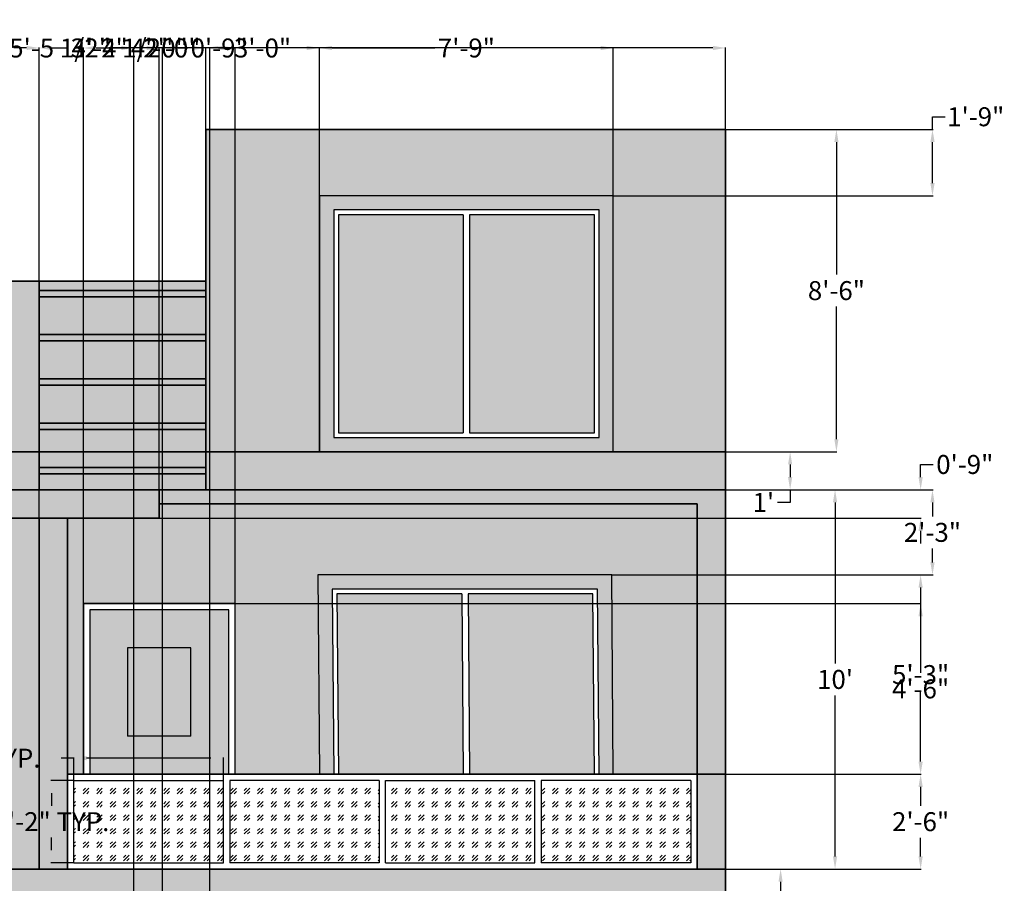
# Model space of a CAD drawing. Units: inches. Extents: x 23 to 640, y 58 to 516.
# Tile 4 of 4: x 328 to 639, y 243 to 516. Entities that reach past the tile are written whole.
import ezdxf

# ---------------------------------------------------------------- set-up
doc = ezdxf.new("R2010")
doc.units = ezdxf.units.IN
doc.header["$MEASUREMENT"] = 0
for name, color, linetype, lineweight in [('A-ANNO-DIMS', 2, 'Continuous', 18), ('A-DOOR', 3, 'Continuous', 25), ('A-ELEV', 7, 'Continuous', 35), ('A-ELEV-PATT', 252, 'Continuous', 13), ('A-GLAZ', 4, 'Continuous', 25)]:
    doc.layers.add(name, color=color, linetype=linetype, lineweight=lineweight)
doc.styles.get("Standard").update_dxf_attribs({"font": 'arial.ttf'})
doc.dimstyles.get("Standard").update_dxf_attribs({"dimtxt": 6, "dimasz": 4, "dimexe": 0.18, "dimexo": 0.0625, "dimgap": 2, "dimtad": 0, "dimtih": 1, "dimtoh": 1, "dimdec": 0, "dimzin": 0, "dimdsep": 46, "dimlunit": 3, "dimtxsty": 'Standard', "dimcen": 2, "dimadec": 0, "dimazin": 0, "dimtfac": 1, "dimtdec": 0, "dimtofl": 0, "dimtmove": 0, "dimatfit": 3, "dimfxl": 1, "dimtolj": 1, "dimtzin": 0, "dimarcsym": 0})

# ---------------------------------------------------------------- blocks, each defined once
blk = doc.blocks.new('*D6')
at = {"layer": 'A-ANNO-DIMS', "color": 0, "lineweight": -2, "transparency": 16777216}
for p, q in [((551.19, 481.68), (586.41, 481.68)), ((586.23, 477.68), (586.23, 435.74)), ((586.23, 383.68), (586.23, 425.62)), ((551.19, 379.68), (586.41, 379.68))]:
    blk.add_line(p, q, dxfattribs=at)
at = {"layer": 'A-ANNO-DIMS', "color": 0, "transparency": 16777216}
for points in [[(585.57, 477.68), (586.9, 477.68), (586.23, 481.68)], [(585.57, 383.68), (586.9, 383.68), (586.23, 379.68)]]:
    blk.add_solid(points, dxfattribs=at)
at = {"layer": 'Defpoints', "color": 0, "transparency": 16777216}
for p in [(551.13, 481.68), (551.13, 379.68), (586.23, 379.68)]:
    blk.add_point(p, dxfattribs=at)
at = {"layer": 'A-ANNO-DIMS', "color": 0, "transparency": 16777216, "insert": (586.23, 430.68), "char_height": 6, "attachment_point": 5}
blk.add_mtext('\\A1;8\'-6"', dxfattribs=at)
blk = doc.blocks.new('*D7')
at = {"layer": 'A-ANNO-DIMS', "color": 0, "lineweight": -2, "transparency": 16777216}
for p, q in [((551.19, 379.68), (571.76, 379.68)), ((571.58, 375.68), (571.58, 371.68)), ((551.19, 367.68), (571.76, 367.68)), ((571.58, 367.68), (571.58, 363.68)), ((571.58, 363.68), (567.58, 363.68))]:
    blk.add_line(p, q, dxfattribs=at)
at = {"layer": 'A-ANNO-DIMS', "color": 0, "transparency": 16777216}
for points in [[(570.92, 375.68), (572.25, 375.68), (571.58, 379.68)], [(570.92, 371.68), (572.25, 371.68), (571.58, 367.68)]]:
    blk.add_solid(points, dxfattribs=at)
at = {"layer": 'Defpoints', "color": 0, "transparency": 16777216}
for p in [(551.13, 379.68), (551.13, 367.68), (571.58, 367.68)]:
    blk.add_point(p, dxfattribs=at)
at = {"layer": 'A-ANNO-DIMS', "color": 0, "transparency": 16777216, "insert": (563.11, 363.68), "char_height": 6, "attachment_point": 5}
blk.add_mtext("\\A1;1'", dxfattribs=at)
blk = doc.blocks.new('*D8')
at = {"layer": 'A-ANNO-DIMS', "color": 0, "lineweight": -2, "transparency": 16777216}
for p, q in [((551.19, 367.68), (585.98, 367.68)), ((585.8, 363.68), (585.8, 312.74)), ((585.8, 251.68), (585.8, 302.62)), ((551.19, 247.68), (585.98, 247.68))]:
    blk.add_line(p, q, dxfattribs=at)
at = {"layer": 'A-ANNO-DIMS', "color": 0, "transparency": 16777216}
for points in [[(585.13, 363.68), (586.47, 363.68), (585.8, 367.68)], [(585.13, 251.68), (586.47, 251.68), (585.8, 247.68)]]:
    blk.add_solid(points, dxfattribs=at)
at = {"layer": 'Defpoints', "color": 0, "transparency": 16777216}
for p in [(551.13, 367.68), (551.13, 247.68), (585.8, 247.68)]:
    blk.add_point(p, dxfattribs=at)
at = {"layer": 'A-ANNO-DIMS', "color": 0, "transparency": 16777216, "insert": (585.8, 307.68), "char_height": 6, "attachment_point": 5}
blk.add_mtext("\\A1;10'", dxfattribs=at)
blk = doc.blocks.new('*D9')
at = {"layer": 'A-ANNO-DIMS', "color": 0, "lineweight": -2, "transparency": 16777216}
for p, q in [((551.19, 247.68), (568.75, 247.68)), ((568.57, 243.68), (568.57, 239.68)), ((551.19, 235.68), (568.75, 235.68)), ((568.57, 235.68), (568.57, 231.68)), ((568.57, 231.68), (564.57, 231.68))]:
    blk.add_line(p, q, dxfattribs=at)
at = {"layer": 'A-ANNO-DIMS', "color": 0, "transparency": 16777216}
for points in [[(567.9, 243.68), (569.23, 243.68), (568.57, 247.68)], [(567.9, 239.68), (569.23, 239.68), (568.57, 235.68)]]:
    blk.add_solid(points, dxfattribs=at)
at = {"layer": 'Defpoints', "color": 0, "transparency": 16777216}
for p in [(551.13, 247.68), (551.13, 235.68), (568.57, 235.68)]:
    blk.add_point(p, dxfattribs=at)
at = {"layer": 'A-ANNO-DIMS', "color": 0, "transparency": 16777216, "insert": (560.09, 231.68), "char_height": 6, "attachment_point": 5}
blk.add_mtext("\\A1;1'", dxfattribs=at)
blk = doc.blocks.new('WIN-SLIDING-2P')
for p, q in [((45.5, 75), (45.5, 6)), ((47.5, 75), (47.5, 6))]:
    blk.add_line(p, q)
for points in [[(93, 81), (0, 81), (0, 0), (93, 0)], [(88.5, 76.5), (4.5, 76.5), (4.5, 4.5), (88.5, 4.5)]]:
    blk.add_lwpolyline(points, close=True)
for points in [[(45.5, 75), (6, 75), (6, 6), (45.5, 6)], [(47.5, 6), (87, 6), (87, 75), (47.5, 75)]]:
    blk.add_lwpolyline(points)
blk = doc.blocks.new('RAIL-GLASS-PANEL')
for p, q in [((47.3, 26), (0, 26)), ((0, 26), (0, 0)), ((47.3, 26), (47.3, 0)), ((47.3, 0), (0, 0))]:
    blk.add_line(p, q)
blk = doc.blocks.new('*D13')
at = {"layer": 'A-ANNO-DIMS', "color": 0, "lineweight": -2, "transparency": 16777216}
for p, q in [((344.93, 282.78), (340.93, 282.78)), ((344.93, 275.74), (344.93, 282.96)), ((388.23, 282.78), (348.93, 282.78)), ((392.23, 275.74), (392.23, 282.96))]:
    blk.add_line(p, q, dxfattribs=at)
at = {"layer": 'A-ANNO-DIMS', "color": 0, "transparency": 16777216}
for points in [[(348.93, 283.44), (348.93, 282.11), (344.93, 282.78)], [(388.23, 283.44), (388.23, 282.11), (392.23, 282.78)]]:
    blk.add_solid(points, dxfattribs=at)
at = {"layer": 'Defpoints', "color": 0, "transparency": 16777216}
for p in [(344.93, 282.78), (344.93, 275.68), (392.23, 275.68)]:
    blk.add_point(p, dxfattribs=at)
at = {"layer": 'A-ANNO-DIMS', "color": 0, "transparency": 16777216, "insert": (263.39, 282.78), "char_height": 6, "attachment_point": 5}
blk.add_mtext('\\A1;GLASS RAILING PANEL 3\'-11 1/2" TYP.', dxfattribs=at)
blk = doc.blocks.new('*D14')
at = {"layer": 'A-ANNO-DIMS', "color": 0, "lineweight": -2, "transparency": 16777216}
for p, q in [((344.87, 275.68), (337.65, 275.68)), ((337.83, 271.68), (337.83, 267.7)), ((337.83, 253.68), (337.83, 257.67)), ((344.87, 249.68), (337.65, 249.68))]:
    blk.add_line(p, q, dxfattribs=at)
at = {"layer": 'A-ANNO-DIMS', "color": 0, "transparency": 16777216}
for points in [[(337.17, 271.68), (338.5, 271.68), (337.83, 275.68)], [(337.17, 253.68), (338.5, 253.68), (337.83, 249.68)]]:
    blk.add_solid(points, dxfattribs=at)
at = {"layer": 'Defpoints', "color": 0, "transparency": 16777216}
for p in [(344.93, 275.68), (337.83, 249.68), (344.93, 249.68)]:
    blk.add_point(p, dxfattribs=at)
at = {"layer": 'A-ANNO-DIMS', "color": 0, "transparency": 16777216, "insert": (337.83, 262.68), "char_height": 6, "attachment_point": 5}
blk.add_mtext('\\A1;2\'-2" TYP.', dxfattribs=at)
blk = doc.blocks.new('*D18')
at = {"layer": 'A-ANNO-DIMS', "color": 0, "lineweight": -2, "transparency": 16777216}
for p, q in [((297.93, 433.74), (297.93, 507.61)), ((301.93, 507.43), (305.96, 507.43)), ((329.93, 507.43), (325.9, 507.43)), ((333.93, 433.74), (333.93, 507.61))]:
    blk.add_line(p, q, dxfattribs=at)
at = {"layer": 'A-ANNO-DIMS', "color": 0, "transparency": 16777216}
for points in [[(301.93, 508.1), (301.93, 506.76), (297.93, 507.43)], [(329.93, 508.1), (329.93, 506.76), (333.93, 507.43)]]:
    blk.add_solid(points, dxfattribs=at)
at = {"layer": 'Defpoints', "color": 0, "transparency": 16777216}
for p in [(333.93, 507.43), (297.93, 433.68), (333.93, 433.68)]:
    blk.add_point(p, dxfattribs=at)
at = {"layer": 'A-ANNO-DIMS', "color": 0, "transparency": 16777216, "insert": (315.93, 507.43), "char_height": 6, "attachment_point": 5}
blk.add_mtext('\\A1;3\'-0"', dxfattribs=at)
blk = doc.blocks.new('*D19')
at = {"layer": 'A-ANNO-DIMS', "color": 0, "lineweight": -2, "transparency": 16777216}
for p, q in [((333.93, 433.74), (333.93, 507.61)), ((337.93, 507.43), (343.19, 507.43)), ((382.63, 507.43), (377.36, 507.43)), ((386.63, 481.74), (386.63, 507.61))]:
    blk.add_line(p, q, dxfattribs=at)
at = {"layer": 'A-ANNO-DIMS', "color": 0, "transparency": 16777216}
for points in [[(337.93, 508.1), (337.93, 506.76), (333.93, 507.43)], [(382.63, 508.1), (382.63, 506.76), (386.63, 507.43)]]:
    blk.add_solid(points, dxfattribs=at)
at = {"layer": 'Defpoints', "color": 0, "transparency": 16777216}
for p in [(386.63, 507.43), (386.63, 481.68), (333.93, 433.68)]:
    blk.add_point(p, dxfattribs=at)
at = {"layer": 'A-ANNO-DIMS', "color": 0, "transparency": 16777216, "insert": (360.28, 507.43), "char_height": 6, "attachment_point": 5}
blk.add_mtext('\\A1;4\'-4 1/2"', dxfattribs=at)
blk = doc.blocks.new('*D20')
at = {"layer": 'A-ANNO-DIMS', "color": 0, "lineweight": -2, "transparency": 16777216}
for p, q in [((386.63, 374.82), (386.63, 507.61)), ((390.63, 507.43), (394.66, 507.43)), ((418.63, 507.43), (414.6, 507.43)), ((422.63, 379.74), (422.63, 507.61))]:
    blk.add_line(p, q, dxfattribs=at)
at = {"layer": 'A-ANNO-DIMS', "color": 0, "transparency": 16777216}
for points in [[(390.63, 508.1), (390.63, 506.76), (386.63, 507.43)], [(418.63, 508.1), (418.63, 506.76), (422.63, 507.43)]]:
    blk.add_solid(points, dxfattribs=at)
at = {"layer": 'Defpoints', "color": 0, "transparency": 16777216}
for p in [(422.63, 507.43), (422.63, 379.68), (386.63, 374.76)]:
    blk.add_point(p, dxfattribs=at)
at = {"layer": 'A-ANNO-DIMS', "color": 0, "transparency": 16777216, "insert": (404.63, 507.43), "char_height": 6, "attachment_point": 5}
blk.add_mtext('\\A1;3\'-0"', dxfattribs=at)
blk = doc.blocks.new('*D21')
at = {"layer": 'A-ANNO-DIMS', "color": 0, "lineweight": -2, "transparency": 16777216}
for p, q in [((422.63, 379.74), (422.63, 507.61)), ((426.63, 507.43), (459.18, 507.43)), ((511.63, 507.43), (479.08, 507.43)), ((515.63, 379.74), (515.63, 507.61))]:
    blk.add_line(p, q, dxfattribs=at)
at = {"layer": 'A-ANNO-DIMS', "color": 0, "transparency": 16777216}
for points in [[(426.63, 508.1), (426.63, 506.76), (422.63, 507.43)], [(511.63, 508.1), (511.63, 506.76), (515.63, 507.43)]]:
    blk.add_solid(points, dxfattribs=at)
at = {"layer": 'Defpoints', "color": 0, "transparency": 16777216}
for p in [(515.63, 507.43), (422.63, 379.68), (515.63, 379.68)]:
    blk.add_point(p, dxfattribs=at)
at = {"layer": 'A-ANNO-DIMS', "color": 0, "transparency": 16777216, "insert": (469.13, 507.43), "char_height": 6, "attachment_point": 5}
blk.add_mtext('\\A1;7\'-9"', dxfattribs=at)
blk = doc.blocks.new('*D22')
at = {"layer": 'A-ANNO-DIMS', "color": 0, "lineweight": -2, "transparency": 16777216}
for p, q in [((125.43, 433.74), (125.43, 507.61)), ((129.43, 507.43), (318.98, 507.43)), ((547.13, 507.43), (357.57, 507.43)), ((551.13, 481.74), (551.13, 507.61))]:
    blk.add_line(p, q, dxfattribs=at)
at = {"layer": 'A-ANNO-DIMS', "color": 0, "transparency": 16777216}
for points in [[(129.43, 508.1), (129.43, 506.76), (125.43, 507.43)], [(547.13, 508.1), (547.13, 506.76), (551.13, 507.43)]]:
    blk.add_solid(points, dxfattribs=at)
at = {"layer": 'Defpoints', "color": 0, "transparency": 16777216}
for p in [(551.13, 507.43), (551.13, 481.68), (125.43, 433.68)]:
    blk.add_point(p, dxfattribs=at)
at = {"layer": 'A-ANNO-DIMS', "color": 0, "transparency": 16777216, "insert": (338.28, 507.43), "char_height": 6, "attachment_point": 5}
blk.add_mtext('\\A1;35\'-5 1/2"', dxfattribs=at)
blk = doc.blocks.new('*D36')
at = {"layer": 'A-ANNO-DIMS', "color": 0, "lineweight": -2, "transparency": 16777216}
for p, q in [((359.93, 507.43), (355.93, 507.43)), ((363.93, 163.74), (363.93, 507.61)), ((387.93, 199.74), (387.93, 507.61)), ((391.93, 507.43), (395.93, 507.43))]:
    blk.add_line(p, q, dxfattribs=at)
at = {"layer": 'A-ANNO-DIMS', "color": 0, "transparency": 16777216}
for points in [[(359.93, 508.1), (359.93, 506.76), (363.93, 507.43)], [(391.93, 508.1), (391.93, 506.76), (387.93, 507.43)]]:
    blk.add_solid(points, dxfattribs=at)
at = {"layer": 'Defpoints', "color": 0, "transparency": 16777216}
for p in [(387.93, 507.43), (387.93, 199.68), (363.93, 163.68)]:
    blk.add_point(p, dxfattribs=at)
at = {"layer": 'A-ANNO-DIMS', "color": 0, "transparency": 16777216, "insert": (375.93, 507.43), "char_height": 6, "attachment_point": 5}
blk.add_mtext('\\A1;2\'-0"', dxfattribs=at)
blk = doc.blocks.new('*D38')
at = {"layer": 'A-ANNO-DIMS', "color": 0, "lineweight": -2, "transparency": 16777216}
for p, q in [((359.93, 507.43), (355.93, 507.43)), ((363.93, 154.74), (363.93, 507.61)), ((372.93, 154.74), (372.93, 507.61)), ((376.93, 507.43), (380.93, 507.43))]:
    blk.add_line(p, q, dxfattribs=at)
at = {"layer": 'A-ANNO-DIMS', "color": 0, "transparency": 16777216}
for points in [[(359.93, 508.1), (359.93, 506.76), (363.93, 507.43)], [(376.93, 508.1), (376.93, 506.76), (372.93, 507.43)]]:
    blk.add_solid(points, dxfattribs=at)
at = {"layer": 'Defpoints', "color": 0, "transparency": 16777216}
for p in [(372.93, 507.43), (363.93, 154.68), (372.93, 154.68)]:
    blk.add_point(p, dxfattribs=at)
at = {"layer": 'A-ANNO-DIMS', "color": 0, "transparency": 16777216, "insert": (390.9, 507.43), "char_height": 6, "attachment_point": 5}
blk.add_mtext('\\A1;0\'-9"', dxfattribs=at)
blk = doc.blocks.new('*D42')
at = {"layer": 'A-ANNO-DIMS', "color": 0, "lineweight": -2, "transparency": 16777216}
for p, q in [((515.21, 340.72), (613.06, 340.72)), ((612.88, 336.72), (612.88, 314.27)), ((612.88, 281.68), (612.88, 304.14)), ((515.69, 277.68), (613.06, 277.68))]:
    blk.add_line(p, q, dxfattribs=at)
at = {"layer": 'A-ANNO-DIMS', "color": 0, "transparency": 16777216}
for points in [[(612.21, 336.72), (613.55, 336.72), (612.88, 340.72)], [(612.21, 281.68), (613.55, 281.68), (612.88, 277.68)]]:
    blk.add_solid(points, dxfattribs=at)
at = {"layer": 'Defpoints', "color": 0, "transparency": 16777216}
for p in [(515.14, 340.72), (612.88, 340.72), (515.63, 277.68)]:
    blk.add_point(p, dxfattribs=at)
at = {"layer": 'A-ANNO-DIMS', "color": 0, "transparency": 16777216, "insert": (612.88, 309.2), "char_height": 6, "attachment_point": 5}
blk.add_mtext('\\A1;5\'-3"', dxfattribs=at)
blk = doc.blocks.new('*D43')
at = {"layer": 'A-ANNO-DIMS', "color": 0, "lineweight": -2, "transparency": 16777216}
for p, q in [((347.93, 331.74), (347.93, 507.61)), ((351.93, 507.43), (361.83, 507.43)), ((391.93, 507.43), (382.02, 507.43)), ((395.93, 331.74), (395.93, 507.61))]:
    blk.add_line(p, q, dxfattribs=at)
at = {"layer": 'A-ANNO-DIMS', "color": 0, "transparency": 16777216}
for points in [[(351.93, 508.1), (351.93, 506.76), (347.93, 507.43)], [(391.93, 508.1), (391.93, 506.76), (395.93, 507.43)]]:
    blk.add_solid(points, dxfattribs=at)
at = {"layer": 'Defpoints', "color": 0, "transparency": 16777216}
for p in [(395.93, 507.43), (347.93, 331.68), (395.93, 331.68)]:
    blk.add_point(p, dxfattribs=at)
at = {"layer": 'A-ANNO-DIMS', "color": 0, "transparency": 16777216, "insert": (371.93, 507.43), "char_height": 6, "attachment_point": 5}
blk.add_mtext('\\A1;4\'-0"', dxfattribs=at)
blk = doc.blocks.new('*D44')
at = {"layer": 'A-ANNO-DIMS', "color": 0, "lineweight": -2, "transparency": 16777216}
for p, q in [((347.99, 331.68), (613.06, 331.68)), ((612.88, 327.68), (612.88, 309.74)), ((612.88, 281.68), (612.88, 299.62)), ((347.99, 277.68), (613.06, 277.68))]:
    blk.add_line(p, q, dxfattribs=at)
at = {"layer": 'A-ANNO-DIMS', "color": 0, "transparency": 16777216}
for points in [[(612.21, 327.68), (613.55, 327.68), (612.88, 331.68)], [(612.21, 281.68), (613.55, 281.68), (612.88, 277.68)]]:
    blk.add_solid(points, dxfattribs=at)
at = {"layer": 'Defpoints', "color": 0, "transparency": 16777216}
for p in [(347.93, 331.68), (612.88, 331.68), (347.93, 277.68)]:
    blk.add_point(p, dxfattribs=at)
at = {"layer": 'A-ANNO-DIMS', "color": 0, "transparency": 16777216, "insert": (612.88, 304.68), "char_height": 6, "attachment_point": 5}
blk.add_mtext('\\A1;4\'-6"', dxfattribs=at)
blk = doc.blocks.new('*D45')
at = {"layer": 'A-ANNO-DIMS', "color": 0, "lineweight": -2, "transparency": 16777216}
for p, q in [((551.19, 277.68), (613.06, 277.68)), ((612.88, 273.68), (612.88, 267.74)), ((612.88, 251.68), (612.88, 257.62)), ((551.19, 247.68), (613.06, 247.68))]:
    blk.add_line(p, q, dxfattribs=at)
at = {"layer": 'A-ANNO-DIMS', "color": 0, "transparency": 16777216}
for points in [[(612.21, 273.68), (613.55, 273.68), (612.88, 277.68)], [(612.21, 251.68), (613.55, 251.68), (612.88, 247.68)]]:
    blk.add_solid(points, dxfattribs=at)
at = {"layer": 'Defpoints', "color": 0, "transparency": 16777216}
for p in [(551.13, 277.68), (612.88, 277.68), (551.13, 247.68)]:
    blk.add_point(p, dxfattribs=at)
at = {"layer": 'A-ANNO-DIMS', "color": 0, "transparency": 16777216, "insert": (612.88, 262.68), "char_height": 6, "attachment_point": 5}
blk.add_mtext('\\A1;2\'-6"', dxfattribs=at)
blk = doc.blocks.new('*D48')
at = {"layer": 'A-ANNO-DIMS', "color": 0, "lineweight": -2, "transparency": 16777216}
for p, q in [((333.93, 358.74), (333.93, 507.61)), ((337.93, 507.43), (342.96, 507.43)), ((367.93, 507.43), (362.9, 507.43)), ((371.93, 358.74), (371.93, 507.61))]:
    blk.add_line(p, q, dxfattribs=at)
at = {"layer": 'A-ANNO-DIMS', "color": 0, "transparency": 16777216}
for points in [[(337.93, 508.1), (337.93, 506.76), (333.93, 507.43)], [(367.93, 508.1), (367.93, 506.76), (371.93, 507.43)]]:
    blk.add_solid(points, dxfattribs=at)
at = {"layer": 'Defpoints', "color": 0, "transparency": 16777216}
for p in [(371.93, 507.43), (333.93, 358.68), (371.93, 358.68)]:
    blk.add_point(p, dxfattribs=at)
at = {"layer": 'A-ANNO-DIMS', "color": 0, "transparency": 16777216, "insert": (352.93, 507.43), "char_height": 6, "attachment_point": 5}
blk.add_mtext('\\A1;3\'-2"', dxfattribs=at)
blk = doc.blocks.new('*D49')
at = {"layer": 'A-ANNO-DIMS', "color": 0, "lineweight": -2, "transparency": 16777216}
for p, q in [((612.88, 371.68), (612.88, 375.68)), ((612.88, 375.68), (616.88, 375.68)), ((371.99, 367.68), (613.06, 367.68)), ((371.99, 358.68), (613.06, 358.68)), ((612.88, 354.68), (612.88, 350.68))]:
    blk.add_line(p, q, dxfattribs=at)
at = {"layer": 'A-ANNO-DIMS', "color": 0, "transparency": 16777216}
for points in [[(612.21, 371.68), (613.55, 371.68), (612.88, 367.68)], [(612.21, 354.68), (613.55, 354.68), (612.88, 358.68)]]:
    blk.add_solid(points, dxfattribs=at)
at = {"layer": 'Defpoints', "color": 0, "transparency": 16777216}
for p in [(371.93, 367.68), (612.88, 367.68), (371.93, 358.68)]:
    blk.add_point(p, dxfattribs=at)
at = {"layer": 'A-ANNO-DIMS', "color": 0, "transparency": 16777216, "insert": (626.85, 375.68), "char_height": 6, "attachment_point": 5}
blk.add_mtext('\\A1;0\'-9"', dxfattribs=at)
blk = doc.blocks.new('*D59')
at = {"layer": 'A-ANNO-DIMS', "color": 0, "lineweight": -2, "transparency": 16777216}
for p, q in [((616.63, 481.68), (616.63, 485.68)), ((616.63, 485.68), (620.63, 485.68)), ((551.19, 481.68), (616.81, 481.68)), ((616.63, 464.68), (616.63, 477.68)), ((515.69, 460.68), (616.81, 460.68))]:
    blk.add_line(p, q, dxfattribs=at)
at = {"layer": 'A-ANNO-DIMS', "color": 0, "transparency": 16777216}
for points in [[(615.96, 477.68), (617.3, 477.68), (616.63, 481.68)], [(615.96, 464.68), (617.3, 464.68), (616.63, 460.68)]]:
    blk.add_solid(points, dxfattribs=at)
at = {"layer": 'Defpoints', "color": 0, "transparency": 16777216}
for p in [(551.13, 481.68), (616.63, 481.68), (515.63, 460.68)]:
    blk.add_point(p, dxfattribs=at)
at = {"layer": 'A-ANNO-DIMS', "color": 0, "transparency": 16777216, "insert": (630.32, 485.68), "char_height": 6, "attachment_point": 5}
blk.add_mtext('\\A1;1\'-9"', dxfattribs=at)
blk = doc.blocks.new('*D60')
at = {"layer": 'A-ANNO-DIMS', "color": 0, "lineweight": -2, "transparency": 16777216}
for p, q in [((551.19, 367.68), (616.81, 367.68)), ((616.63, 363.68), (616.63, 359.27)), ((616.63, 344.72), (616.63, 349.14)), ((515.21, 340.72), (616.81, 340.72))]:
    blk.add_line(p, q, dxfattribs=at)
at = {"layer": 'A-ANNO-DIMS', "color": 0, "transparency": 16777216}
for points in [[(615.96, 363.68), (617.3, 363.68), (616.63, 367.68)], [(615.96, 344.72), (617.3, 344.72), (616.63, 340.72)]]:
    blk.add_solid(points, dxfattribs=at)
at = {"layer": 'Defpoints', "color": 0, "transparency": 16777216}
for p in [(551.13, 367.68), (616.63, 367.68), (515.14, 340.72)]:
    blk.add_point(p, dxfattribs=at)
at = {"layer": 'A-ANNO-DIMS', "color": 0, "transparency": 16777216, "insert": (616.63, 354.2), "char_height": 6, "attachment_point": 5}
blk.add_mtext('\\A1;2\'-3"', dxfattribs=at)

msp = doc.modelspace()

# ---------------------------------------------------------------- hatches: boundary and pattern name
at = {"layer": 'A-ELEV-PATT'}
h = msp.add_hatch(color=256, dxfattribs=at)
h.set_gradient(color1=(255, 255, 255), color2=(199, 200, 202), name='INVCYLINDER')
h.paths.add_polyline_path([(515.63, 379.68), (551.13, 379.68), (551.13, 481.68), (386.63, 481.68), (386.63, 379.68), (422.63, 379.68), (422.63, 460.68), (515.63, 460.68)])
h.paths.add_polyline_path([(386.63, 379.68), (386.63, 367.68), (551.13, 367.68), (551.13, 379.68)])
h = msp.add_hatch(color=256, dxfattribs=at)
h.set_gradient(color1=(153, 76, 76), color2=(147, 149, 152), name='SPHERICAL')
h.paths.add_polyline_path([(422.63, 379.68), (515.63, 379.68), (515.63, 460.68), (422.63, 460.68)])
h.paths.add_polyline_path([(427.13, 456.18), (511.13, 456.18), (511.13, 384.18), (427.13, 384.18)], flags=16)
h.paths.add_polyline_path([(428.63, 454.68), (468.13, 454.68), (468.13, 385.68), (428.63, 385.68)], flags=0)
h.paths.add_polyline_path([(470.13, 454.68), (509.63, 454.68), (509.63, 385.68), (470.13, 385.68)], flags=0)
h = msp.add_hatch(color=256, dxfattribs=at)
h.set_gradient(color1=(255, 255, 255), color2=(173, 221, 247), name='INVSPHERICAL')
h.paths.add_polyline_path([(468.13, 454.68), (428.63, 454.68), (428.63, 385.68), (468.13, 385.68)])
h = msp.add_hatch(color=256, dxfattribs=at)
h.set_gradient(color1=(255, 255, 255), color2=(173, 221, 247), name='INVSPHERICAL')
h.paths.add_polyline_path([(509.63, 454.68), (470.13, 454.68), (470.13, 385.68), (509.63, 385.68)])
h = msp.add_hatch(color=256, dxfattribs=at)
h.dxf.hatch_style = 1
h.paths.add_polyline_path([(180.93, 120.76), (125.43, 120.76), (125.43, 115.68), (180.93, 115.68)])
h.paths.add_polyline_path([(180.93, 134.76), (125.43, 134.76), (125.43, 122.76), (180.93, 122.76)])
h.paths.add_polyline_path([(180.93, 148.76), (125.43, 148.76), (125.43, 136.76), (180.93, 136.76)])
h.paths.add_polyline_path([(180.93, 162.76), (125.43, 162.76), (125.43, 150.76), (180.93, 150.76)])
h.paths.add_polyline_path([(180.93, 176.76), (125.43, 176.76), (125.43, 164.76), (180.93, 164.76)])
h.paths.add_polyline_path([(180.93, 190.76), (125.43, 190.76), (125.43, 178.76), (180.93, 178.76)])
h.paths.add_polyline_path([(180.93, 204.76), (125.43, 204.76), (125.43, 192.76), (180.93, 192.76)])
h.paths.add_polyline_path([(180.93, 218.76), (125.43, 218.76), (125.43, 206.76), (180.93, 206.76)])
h.paths.add_polyline_path([(180.93, 232.76), (125.43, 232.76), (125.43, 220.76), (180.93, 220.76)])
h.paths.add_polyline_path([(180.93, 246.76), (125.43, 246.76), (125.43, 235.68), (180.93, 235.68)])
h.paths.add_polyline_path([(180.93, 235.68), (125.43, 235.68), (125.43, 234.76), (180.93, 234.76)])
h.paths.add_polyline_path([(180.93, 260.76), (125.43, 260.76), (125.43, 248.76), (180.93, 248.76)])
h.paths.add_polyline_path([(180.93, 274.76), (125.43, 274.76), (125.43, 262.76), (180.93, 262.76)])
h.paths.add_polyline_path([(180.93, 288.76), (125.43, 288.76), (125.43, 276.76), (180.93, 276.76)])
h.paths.add_polyline_path([(180.93, 302.76), (125.43, 302.76), (125.43, 290.76), (180.93, 290.76)])
h.paths.add_polyline_path([(180.93, 316.76), (125.43, 316.76), (125.43, 304.76), (180.93, 304.76)])
h.paths.add_polyline_path([(180.93, 330.76), (125.43, 330.76), (125.43, 318.76), (180.93, 318.76)])
h.paths.add_polyline_path([(180.93, 344.76), (125.43, 344.76), (125.43, 332.76), (180.93, 332.76)])
h.paths.add_polyline_path([(180.93, 358.76), (125.43, 358.76), (125.43, 346.76), (180.93, 346.76)])
h.paths.add_polyline_path([(180.93, 367.68), (125.43, 367.68), (125.43, 360.76), (180.93, 360.76)])
h.paths.add_polyline_path([(297.93, 372.76), (125.43, 372.76), (125.43, 367.68), (180.93, 367.68), (297.93, 367.68)])
h.paths.add_polyline_path([(297.93, 379.68), (125.43, 379.68), (125.43, 374.76), (297.93, 374.76)])
h.paths.add_polyline_path([(297.93, 386.76), (125.43, 386.76), (125.43, 379.68), (297.93, 379.68)])
h.paths.add_polyline_path([(297.93, 400.76), (125.43, 400.76), (125.43, 388.76), (297.93, 388.76)])
h.paths.add_polyline_path([(297.93, 414.76), (125.43, 414.76), (125.43, 402.76), (297.93, 402.76)])
h.paths.add_polyline_path([(297.93, 433.68), (125.43, 433.68), (125.43, 430.76), (297.93, 430.76)])
h.paths.add_polyline_path([(386.63, 372.76), (333.93, 372.76), (333.93, 367.68), (386.63, 367.68)])
h.paths.add_polyline_path([(386.63, 379.68), (333.93, 379.68), (333.93, 374.76), (386.63, 374.76)])
h.paths.add_polyline_path([(386.63, 386.76), (333.93, 386.76), (333.93, 379.68), (386.63, 379.68)])
h.paths.add_polyline_path([(386.63, 400.76), (333.93, 400.76), (333.93, 388.76), (386.63, 388.76)])
h.paths.add_polyline_path([(386.63, 414.76), (333.93, 414.76), (333.93, 402.76), (386.63, 402.76)])
h.paths.add_polyline_path([(386.63, 428.76), (333.93, 428.76), (333.93, 416.76), (386.63, 416.76)])
h.paths.add_polyline_path([(386.63, 433.68), (333.93, 433.68), (333.93, 430.76), (386.63, 430.76)])
h = msp.add_hatch(color=256, dxfattribs=at)
h.dxf.hatch_style = 1
h.paths.add_polyline_path([(333.93, 433.68), (297.93, 433.68), (297.93, 379.68), (333.93, 379.68)])
h.paths.add_polyline_path([(333.93, 379.68), (297.93, 379.68), (297.93, 367.68), (333.93, 367.68)])
h.paths.add_polyline_path([(333.93, 358.68), (297.93, 358.68), (297.93, 247.68), (333.93, 247.68)])
h.paths.add_polyline_path([(333.93, 229.68), (297.93, 229.68), (297.93, 215.06), (333.93, 215.06)])
h.paths.add_polyline_path([(333.93, 206.06), (297.93, 206.06), (297.93, 115.68), (333.93, 115.68)])
h = msp.add_hatch(color=256, dxfattribs=at)
h.dxf.hatch_style = 1
h.paths.add_polyline_path([(180.93, 122.76), (125.43, 122.76), (125.43, 120.76), (180.93, 120.76)])
h.paths.add_polyline_path([(180.93, 136.76), (125.43, 136.76), (125.43, 134.76), (180.93, 134.76)])
h.paths.add_polyline_path([(180.93, 150.76), (125.43, 150.76), (125.43, 148.76), (180.93, 148.76)])
h.paths.add_polyline_path([(180.93, 164.76), (125.43, 164.76), (125.43, 162.76), (180.93, 162.76)])
h.paths.add_polyline_path([(180.93, 178.76), (125.43, 178.76), (125.43, 176.76), (180.93, 176.76)])
h.paths.add_polyline_path([(180.93, 192.76), (125.43, 192.76), (125.43, 190.76), (180.93, 190.76)])
h.paths.add_polyline_path([(180.93, 206.76), (125.43, 206.76), (125.43, 204.76), (180.93, 204.76)])
h.paths.add_polyline_path([(180.93, 220.76), (125.43, 220.76), (125.43, 218.76), (180.93, 218.76)])
h.paths.add_polyline_path([(180.93, 234.76), (125.43, 234.76), (125.43, 232.76), (180.93, 232.76)])
h.paths.add_polyline_path([(180.93, 247.68), (125.43, 247.68), (125.43, 246.76), (180.93, 246.76)])
h.paths.add_polyline_path([(180.93, 248.76), (125.43, 248.76), (125.43, 247.68), (180.93, 247.68)])
h.paths.add_polyline_path([(180.93, 262.76), (125.43, 262.76), (125.43, 260.76), (180.93, 260.76)])
h.paths.add_polyline_path([(180.93, 276.76), (125.43, 276.76), (125.43, 274.76), (180.93, 274.76)])
h.paths.add_polyline_path([(180.93, 290.76), (125.43, 290.76), (125.43, 288.76), (180.93, 288.76)])
h.paths.add_polyline_path([(180.93, 304.76), (125.43, 304.76), (125.43, 302.76), (180.93, 302.76)])
h.paths.add_polyline_path([(180.93, 318.76), (125.43, 318.76), (125.43, 316.76), (180.93, 316.76)])
h.paths.add_polyline_path([(180.93, 332.76), (125.43, 332.76), (125.43, 330.76), (180.93, 330.76)])
h.paths.add_polyline_path([(180.93, 346.76), (125.43, 346.76), (125.43, 344.76), (180.93, 344.76)])
h.paths.add_polyline_path([(180.93, 360.76), (125.43, 360.76), (125.43, 358.76), (180.93, 358.76)])
h.paths.add_polyline_path([(297.93, 374.76), (125.43, 374.76), (125.43, 372.76), (297.93, 372.76)])
h.paths.add_polyline_path([(297.93, 388.76), (125.43, 388.76), (125.43, 386.76), (297.93, 386.76)])
h.paths.add_polyline_path([(297.93, 402.76), (125.43, 402.76), (125.43, 400.76), (297.93, 400.76)])
h.paths.add_polyline_path([(297.93, 416.76), (125.43, 416.76), (125.43, 414.76), (297.93, 414.76)])
h.paths.add_polyline_path([(297.93, 430.76), (125.43, 430.76), (125.43, 428.76), (297.93, 428.76)])
h.paths.add_polyline_path([(386.63, 374.76), (333.93, 374.76), (333.93, 372.76), (386.63, 372.76)])
h.paths.add_polyline_path([(386.63, 388.76), (333.93, 388.76), (333.93, 386.76), (386.63, 386.76)])
h.paths.add_polyline_path([(386.63, 402.76), (333.93, 402.76), (333.93, 400.76), (386.63, 400.76)])
h.paths.add_polyline_path([(386.63, 416.76), (333.93, 416.76), (333.93, 414.76), (386.63, 414.76)])
h.paths.add_polyline_path([(386.63, 430.76), (333.93, 430.76), (333.93, 428.76), (386.63, 428.76)])
h = msp.add_hatch(color=256, dxfattribs=at)
h.dxf.hatch_style = 1
h.paths.add_polyline_path([(371.93, 367.68), (180.93, 367.68), (180.93, 247.68), (189.93, 247.68), (189.93, 358.68), (371.93, 358.68)])
h.paths.add_polyline_path([(189.93, 247.68), (180.93, 247.68), (180.93, 235.68), (189.93, 235.68)])
h.paths.add_polyline_path([(189.93, 235.68), (180.93, 235.68), (180.93, 206.06), (333.93, 206.06), (351.93, 206.06), (351.93, 211.68), (351.93, 215.06), (189.93, 215.06)])
h.paths.add_polyline_path([(551.13, 247.68), (280.13, 247.68), (280.13, 235.68), (551.13, 235.68)])
h.paths.add_polyline_path([(551.13, 235.68), (280.13, 235.68), (280.13, 229.68), (551.13, 229.68)])
h = msp.add_hatch(color=256, dxfattribs=at)
h.dxf.hatch_style = 1
h.paths.add_polyline_path([(551.13, 367.68), (371.93, 367.68), (371.93, 363.18), (542.13, 363.18), (542.13, 277.68), (551.13, 277.68)])
h = msp.add_hatch(color=256, dxfattribs=at)
h.set_gradient(color1=(255, 255, 255), color2=(199, 200, 202), name='INVCYLINDER')
h.paths.add_polyline_path([(371.93, 363.18), (371.93, 358.68), (342.93, 358.68), (342.93, 277.68), (347.93, 277.68), (347.93, 331.68), (395.93, 331.68), (395.93, 277.68), (422.63, 277.68), (422.14, 340.72), (515.14, 340.72), (515.63, 277.68), (542.13, 277.68), (542.13, 363.18)])
h = msp.add_hatch(color=256, dxfattribs=at)
h.set_gradient(color1=(147, 149, 152), color2=(199, 200, 202), name='INVCYLINDER')
h.paths.add_polyline_path([(342.93, 358.68), (333.93, 358.68), (333.93, 247.68), (342.93, 247.68)])
h = msp.add_hatch(color=256, dxfattribs=at)
h.set_gradient(color1=(153, 76, 76), color2=(147, 149, 152), name='SPHERICAL')
h.paths.add_polyline_path([(422.63, 277.68), (427.13, 277.68), (426.64, 336.22), (510.64, 336.22), (511.13, 277.68), (515.63, 277.68), (515.14, 340.72), (422.14, 340.72)])
h = msp.add_hatch(color=256, dxfattribs=at)
h.set_gradient(color1=(255, 255, 255), color2=(173, 221, 247), name='INVSPHERICAL')
h.paths.add_polyline_path([(428.63, 277.68), (468.13, 277.68), (467.64, 334.72), (428.14, 334.72)])
h = msp.add_hatch(color=256, dxfattribs=at)
h.set_gradient(color1=(255, 255, 255), color2=(173, 221, 247), name='INVSPHERICAL')
h.paths.add_polyline_path([(470.13, 277.68), (509.63, 277.68), (509.14, 334.72), (469.64, 334.72)])
h = msp.add_hatch(color=256, dxfattribs=at)
h.set_gradient(color1=(255, 255, 255), color2=(147, 149, 152), name='SPHERICAL')
h.paths.add_polyline_path([(349.93, 277.68), (393.93, 277.68), (393.93, 329.68), (349.93, 329.68)])
h.paths.add_polyline_path([(361.93, 289.68), (361.93, 317.68), (381.93, 317.68), (381.93, 289.68)], flags=16)
h = msp.add_hatch(color=256, dxfattribs=at)
h.set_gradient(color1=(255, 255, 255), color2=(147, 149, 152), name='CYLINDER')
h.paths.add_polyline_path([(381.93, 317.68), (361.93, 317.68), (361.93, 289.68), (381.93, 289.68)])
h = msp.add_hatch(color=256, dxfattribs=at)
h.set_gradient(color1=(147, 149, 152), color2=(99, 100, 102), name='CYLINDER')
h.paths.add_polyline_path([(381.93, 317.68), (361.93, 317.68), (361.93, 289.68), (381.93, 289.68)])
h = msp.add_hatch(color=256, dxfattribs=at)
h.set_gradient(color1=(255, 255, 255), color2=(147, 149, 152), name='HEMISPHERICAL')
h.paths.add_polyline_path([(551.13, 277.68), (542.13, 277.68), (542.13, 247.68), (551.13, 247.68)])
h = msp.add_hatch(dxfattribs=at)
h.set_pattern_fill('GOST_GLASS', color=256, scale=0.5, style=0)
h.set_pattern_definition([(45, (0, 0), (4.24264, 0), [2.5, -3.5]), (45, (1.0607, 0), (4.24264, 0), [1, -5]), (45, (0, 1.0607), (4.24264, 0), [1, -5])])
h.paths.add_polyline_path([(392.23, 275.68), (344.93, 275.68), (344.93, 249.68), (392.23, 249.68)])
h.paths.add_polyline_path([(441.53, 275.68), (394.23, 275.68), (394.23, 249.68), (441.53, 249.68)])
h.paths.add_polyline_path([(490.83, 275.68), (443.53, 275.68), (443.53, 249.68), (490.83, 249.68)])
h.paths.add_polyline_path([(540.13, 275.68), (492.83, 275.68), (492.83, 249.68), (540.13, 249.68)])

# ---------------------------------------------------------------- linework, layer by layer
at = {"layer": 'A-DOOR'}
for p, q in [((395.93, 277.68), (395.93, 331.68)), ((393.93, 329.68), (349.93, 329.68)), ((349.93, 329.68), (349.93, 277.68)), ((393.93, 277.68), (393.93, 329.68)), ((381.93, 317.68), (361.93, 317.68)), ((361.93, 317.68), (361.93, 289.68)), ((381.93, 289.68), (381.93, 317.68)), ((381.93, 289.68), (361.93, 289.68))]:
    msp.add_line(p, q, dxfattribs=at)
at = {"layer": 'A-ELEV'}
for p, q in [((551.13, 481.68), (386.63, 481.68)), ((386.63, 481.68), (386.63, 367.68)), ((551.13, 379.68), (551.13, 481.68)), ((125.43, 433.68), (386.63, 433.68)), ((333.93, 433.68), (333.93, 367.68)), ((333.93, 430.76), (386.63, 430.76)), ((333.93, 428.76), (386.63, 428.76)), ((333.93, 416.76), (386.63, 416.76)), ((333.93, 414.76), (386.63, 414.76)), ((333.93, 402.76), (386.63, 402.76)), ((333.93, 400.76), (386.63, 400.76)), ((333.93, 388.76), (386.63, 388.76)), ((333.93, 386.76), (386.63, 386.76)), ((125.43, 379.68), (551.13, 379.68)), ((551.13, 379.68), (551.13, 115.68)), ((333.93, 374.76), (386.63, 374.76)), ((333.93, 372.76), (386.63, 372.76)), ((125.43, 367.68), (551.13, 367.68)), ((180.93, 367.68), (551.13, 367.68)), ((371.93, 358.68), (371.93, 367.68)), ((371.93, 363.18), (542.13, 363.18)), ((542.13, 277.68), (542.13, 363.18)), ((189.93, 358.68), (371.93, 358.68)), ((333.93, 358.68), (333.93, 247.68)), ((342.93, 358.68), (342.93, 247.68)), ((347.93, 331.68), (347.93, 277.68)), ((395.93, 331.68), (347.93, 331.68)), ((347.93, 331.68), (347.93, 277.68)), ((551.13, 277.68), (342.93, 277.68)), ((347.93, 277.68), (395.93, 277.68)), ((542.13, 277.68), (542.13, 247.68)), ((551.13, 247.68), (551.13, 277.68)), ((125.43, 247.68), (551.13, 247.68)), ((280.13, 247.68), (551.13, 247.68))]:
    msp.add_line(p, q, dxfattribs=at)
at = {"layer": 'A-GLAZ'}
for p, q in [((467.64, 334.72), (468.13, 277.68)), ((469.64, 334.72), (470.13, 277.68)), ((468.13, 277.68), (470.13, 277.68)), ((468.13, 277.68), (470.13, 277.68))]:
    msp.add_line(p, q, dxfattribs=at)
for points in [[(515.63, 277.68), (515.14, 340.72), (422.14, 340.72), (422.63, 277.68)], [(511.13, 277.68), (510.64, 336.22), (426.64, 336.22), (427.13, 277.68)], [(467.64, 334.72), (428.14, 334.72), (428.63, 277.68)], [(509.63, 277.68), (509.14, 334.72), (469.64, 334.72)]]:
    msp.add_lwpolyline(points, dxfattribs=at)

# ---------------------------------------------------------------- block references
for name, p in [('WIN-SLIDING-2P', (422.63, 379.68)), ('RAIL-GLASS-PANEL', (394.23, 249.68)), ('RAIL-GLASS-PANEL', (492.83, 249.68))]:
    msp.add_blockref(name, p, dxfattribs=at)
at = {"layer": 'A-GLAZ', "rotation": 180}
for p in [(392.23, 275.68), (490.83, 275.68)]:
    msp.add_blockref('RAIL-GLASS-PANEL', p, dxfattribs=at)

# ---------------------------------------------------------------- dimensions: what is measured, and where the dimension line sits
at = {"layer": 'A-ANNO-DIMS'}
for base, p1, p2, picture, middle in [((551.13, 507.43), (125.43, 433.68), (551.13, 481.68), '*D22', (338.28, 507.43)), ((386.63, 507.43), (333.93, 433.68), (386.63, 481.68), '*D19', (360.28, 507.43)), ((333.93, 507.43), (297.93, 433.68), (333.93, 433.68), '*D18', (315.93, 507.43)), ((371.93, 507.43), (333.93, 358.68), (371.93, 358.68), '*D48', (352.93, 507.43)), ((395.93, 507.43), (347.93, 331.68), (395.93, 331.68), '*D43', (371.93, 507.43)), ((387.93, 507.43), (363.93, 163.68), (387.93, 199.68), '*D36', (375.93, 507.43)), ((372.93, 507.43), (363.93, 154.68), (372.93, 154.68), '*D38', (390.9, 507.43)), ((422.63, 507.43), (386.63, 374.76), (422.63, 379.68), '*D20', (404.63, 507.43)), ((515.63, 507.43), (422.63, 379.68), (515.63, 379.68), '*D21', (469.13, 507.43))]:
    dim = msp.add_linear_dim(base=base, p1=p1, p2=p2, dimstyle='Standard', override={"dimdec": 1, "dimlfac": 1, "dimrnd": 0, "dimzin": 1, "dimdsep": 46, "dimlunit": 4, "dimfrac": 2}, dxfattribs=at)
    dim.commit()
    dim.dimension.update_dxf_attribs({"geometry": picture, "text_midpoint": middle})
for base, p1, p2, override, picture, middle in [((616.63, 481.68), (515.63, 460.68), (551.13, 481.68), {"dimdec": 1, "dimlfac": 1, "dimrnd": 0, "dimzin": 1, "dimdsep": 46, "dimlunit": 4, "dimfrac": 2}, '*D59', (630.32, 485.68)), ((586.23, 379.68), (551.13, 481.68), (551.13, 379.68), {"dimclrd": 0, "dimclre": 0, "dimclrt": 0}, '*D6', (586.23, 430.68)), ((612.88, 367.68), (371.93, 358.68), (371.93, 367.68), {"dimdec": 1, "dimlfac": 1, "dimrnd": 0, "dimzin": 1, "dimdsep": 46, "dimlunit": 4, "dimfrac": 2}, '*D49', (626.85, 375.68)), ((571.58, 367.68), (551.13, 379.68), (551.13, 367.68), {"dimclrd": 0, "dimclre": 0, "dimclrt": 0}, '*D7', (563.11, 363.68)), ((616.63, 367.68), (515.14, 340.72), (551.13, 367.68), {"dimdec": 1, "dimlfac": 1, "dimrnd": 0, "dimzin": 1, "dimdsep": 46, "dimlunit": 4, "dimfrac": 2}, '*D60', (616.63, 354.2)), ((585.8, 247.68), (551.13, 367.68), (551.13, 247.68), {"dimclrd": 0, "dimclre": 0, "dimclrt": 0}, '*D8', (585.8, 307.68)), ((612.88, 340.72), (515.63, 277.68), (515.14, 340.72), {"dimdec": 1, "dimlfac": 1, "dimrnd": 0, "dimzin": 1, "dimdsep": 46, "dimlunit": 4, "dimfrac": 2}, '*D42', (612.88, 309.2)), ((612.88, 331.68), (347.93, 277.68), (347.93, 331.68), {"dimdec": 1, "dimlfac": 1, "dimrnd": 0, "dimzin": 1, "dimdsep": 46, "dimlunit": 4, "dimfrac": 2}, '*D44', (612.88, 304.68)), ((612.88, 277.68), (551.13, 247.68), (551.13, 277.68), {"dimdec": 1, "dimlfac": 1, "dimrnd": 0, "dimzin": 1, "dimdsep": 46, "dimlunit": 4, "dimfrac": 2}, '*D45', (612.88, 262.68)), ((568.57, 235.68), (551.13, 247.68), (551.13, 235.68), {"dimclrd": 0, "dimclre": 0, "dimclrt": 0}, '*D9', (560.09, 231.68))]:
    dim = msp.add_linear_dim(base=base, p1=p1, p2=p2, angle=90, dimstyle='Standard', override=override, dxfattribs=at)
    dim.commit()
    dim.dimension.update_dxf_attribs({"geometry": picture, "text_midpoint": middle})
for base, p1, p2, angle, text, picture, middle in [((344.93, 282.78), (392.23, 275.68), (344.93, 275.68), 180, 'GLASS RAILING PANEL <> TYP.', '*D13', (263.39, 282.78)), ((337.83, 249.68), (344.93, 275.68), (344.93, 249.68), 270, '<> TYP.', '*D14', (337.83, 262.68))]:
    dim = msp.add_linear_dim(base=base, p1=p1, p2=p2, angle=angle, text=text, dimstyle='Standard', override={"dimdec": 1, "dimrnd": 0, "dimzin": 1, "dimlunit": 4, "dimfrac": 2}, dxfattribs=at)
    dim.commit()
    dim.dimension.update_dxf_attribs({"geometry": picture, "text_midpoint": middle})

doc.saveas('drawing.dxf')
